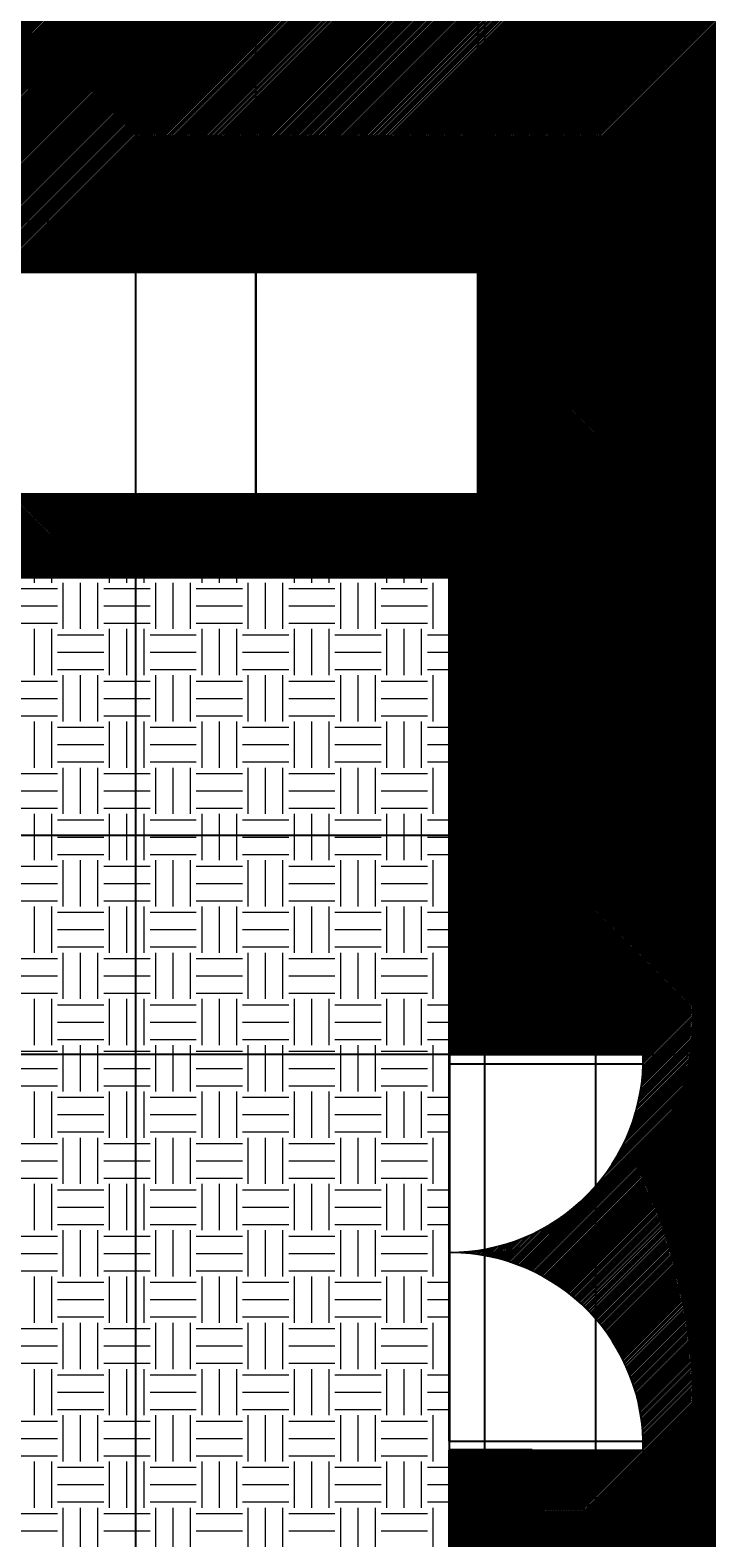
# Model space of a CAD drawing. Units: inches. Extents: x 205 to 1667, y -23 to 828.
# Tile 3 of 10: x 572 to 645, y 101 to 264. Entities that reach past the tile are written whole.
import ezdxf

# ---------------------------------------------------------------- set-up
doc = ezdxf.new("R2010")
doc.units = ezdxf.units.IN
doc.header["$MEASUREMENT"] = 0
for name, color, linetype, lineweight in [('A-ANNO-DIMS', 2, 'Continuous', 18), ('A-DOOR', 4, 'Continuous', 25), ('A-FLOR-CASE', 32, 'Continuous', 25), ('A-WALL', 7, 'Continuous', 35)]:
    doc.layers.add(name, color=color, linetype=linetype, lineweight=lineweight)
doc.layers.add('A-FLOR-PATT', color=9, linetype='Continuous', lineweight=9, true_color=0xc7c8ca)
doc.styles.get("Standard").update_dxf_attribs({"font": 'arial.ttf'})
doc.dimstyles.get("Standard").update_dxf_attribs({"dimtxt": 0.18, "dimasz": 0.18, "dimexe": 0.18, "dimexo": 0.0625, "dimgap": 0.09, "dimtad": 0, "dimtih": 1, "dimtoh": 1, "dimdec": 4, "dimzin": 0, "dimdsep": 46, "dimtxsty": 'Standard', "dimcen": 0.09, "dimadec": 0, "dimazin": 0, "dimtfac": 1, "dimtdec": 4, "dimtofl": 0, "dimtmove": 0, "dimatfit": 3, "dimfxl": 1, "dimtolj": 1, "dimtzin": 0, "dimarcsym": 0})

# ---------------------------------------------------------------- blocks, each defined once
blk = doc.blocks.new('DOOR-PAIR-21IN-LEAVES')
for p, q in [((0, 42.78), (0, 41.78)), ((0, 42.78), (21, 42.78)), ((0, 41.78), (21, 41.78)), ((0, 1), (0, 0)), ((0, 1), (21, 1)), ((0, 0), (21, 0))]:
    blk.add_line(p, q)
for centre, start, end in [((0.11, 42.28), 269.6873, 1.3714), ((0.11, 0.5), 358.6286, 89.6873)]:
    blk.add_arc(centre, 20.89, start, end)
blk = doc.blocks.new('*D19')
at = {"layer": 'A-ANNO-DIMS', "color": 0, "lineweight": -2, "transparency": 16777216}
for p, q in [((570, 213.93), (577.32, 213.93)), ((577.14, 213.75), (577.14, 209.61)), ((577.14, 205.11), (577.14, 209.25)), ((570, 204.93), (577.32, 204.93))]:
    blk.add_line(p, q, dxfattribs=at)
at = {"layer": 'A-ANNO-DIMS', "color": 0, "transparency": 16777216}
for points in [[(577.11, 213.75), (577.17, 213.75), (577.14, 213.93)], [(577.11, 205.11), (577.17, 205.11), (577.14, 204.93)]]:
    blk.add_solid(points, dxfattribs=at)
at = {"layer": 'Defpoints', "color": 0, "transparency": 16777216}
for p in [(569.94, 213.93), (577.14, 213.93), (569.94, 204.93)]:
    blk.add_point(p, dxfattribs=at)
at = {"layer": 'A-ANNO-DIMS', "color": 0, "transparency": 16777216, "insert": (577.14, 209.43), "char_height": 0.18, "attachment_point": 5}
blk.add_mtext('\\A1;9 TYP.', dxfattribs=at)
blk = doc.blocks.new('*D34')
at = {"layer": 'A-ANNO-DIMS', "color": 0, "lineweight": -2, "transparency": 16777216}
for p, q in [((638.54, 153.38), (645.08, 153.38)), ((644.9, 153.2), (644.9, 132.17)), ((644.9, 110.77), (644.9, 131.8)), ((638.54, 110.59), (645.08, 110.59))]:
    blk.add_line(p, q, dxfattribs=at)
at = {"layer": 'A-ANNO-DIMS', "color": 0, "transparency": 16777216}
for points in [[(644.87, 153.2), (644.93, 153.2), (644.9, 153.38)], [(644.87, 110.77), (644.93, 110.77), (644.9, 110.59)]]:
    blk.add_solid(points, dxfattribs=at)
at = {"layer": 'Defpoints', "color": 0, "transparency": 16777216}
for p in [(638.48, 153.38), (644.9, 153.38), (638.48, 110.59)]:
    blk.add_point(p, dxfattribs=at)
at = {"layer": 'A-ANNO-DIMS', "color": 0, "transparency": 16777216, "insert": (644.9, 131.98), "char_height": 0.18, "attachment_point": 5}
blk.add_mtext('\\A1;PAIRED DOOR 43', dxfattribs=at)
blk = doc.blocks.new('*D35')
at = {"layer": 'A-ANNO-DIMS', "color": 0, "lineweight": -2, "transparency": 16777216}
for p, q in [((617.35, 110.53), (617.35, 103.99)), ((638.48, 110.53), (638.48, 103.99)), ((617.53, 104.17), (627.71, 104.17)), ((638.3, 104.17), (628.12, 104.17))]:
    blk.add_line(p, q, dxfattribs=at)
at = {"layer": 'A-ANNO-DIMS', "color": 0, "transparency": 16777216}
for points in [[(617.53, 104.2), (617.53, 104.14), (617.35, 104.17)], [(638.3, 104.2), (638.3, 104.14), (638.48, 104.17)]]:
    blk.add_solid(points, dxfattribs=at)
at = {"layer": 'Defpoints', "color": 0, "transparency": 16777216}
for p in [(617.35, 110.59), (638.48, 110.59), (638.48, 104.17)]:
    blk.add_point(p, dxfattribs=at)
at = {"layer": 'A-ANNO-DIMS', "color": 0, "transparency": 16777216, "insert": (627.91, 104.17), "char_height": 0.18, "attachment_point": 5}
blk.add_mtext('\\A1;21', dxfattribs=at)
blk = doc.blocks.new('*D55')
at = {"layer": 'A-ANNO-DIMS', "color": 0, "lineweight": -2, "transparency": 16777216}
for p, q in [((621.22, 16.71), (621.22, 637.89)), ((621.4, 637.71), (627.01, 637.71)), ((633.04, 637.71), (627.43, 637.71)), ((633.22, 16.71), (633.22, 637.89))]:
    blk.add_line(p, q, dxfattribs=at)
at = {"layer": 'A-ANNO-DIMS', "color": 0, "transparency": 16777216}
for points in [[(621.4, 637.74), (621.4, 637.68), (621.22, 637.71)], [(633.04, 637.74), (633.04, 637.68), (633.22, 637.71)]]:
    blk.add_solid(points, dxfattribs=at)
at = {"layer": 'Defpoints', "color": 0, "transparency": 16777216}
for p in [(633.22, 637.71), (621.22, 16.65), (633.22, 16.65)]:
    blk.add_point(p, dxfattribs=at)
at = {"layer": 'A-ANNO-DIMS', "color": 0, "transparency": 16777216, "insert": (627.22, 637.71), "char_height": 0.18, "attachment_point": 5}
blk.add_mtext('\\A1;12', dxfattribs=at)
blk = doc.blocks.new('*D64')
at = {"layer": 'A-ANNO-DIMS', "color": 0, "lineweight": -2, "transparency": 16777216}
for p, q in [((471.43, 454.59), (471.43, -22.59)), ((583.44, 454.59), (583.44, -22.59)), ((471.61, -22.41), (527.16, -22.41)), ((583.26, -22.41), (527.71, -22.41))]:
    blk.add_line(p, q, dxfattribs=at)
at = {"layer": 'A-ANNO-DIMS', "color": 0, "transparency": 16777216}
for points in [[(471.61, -22.38), (471.61, -22.44), (471.43, -22.41)], [(583.26, -22.38), (583.26, -22.44), (583.44, -22.41)]]:
    blk.add_solid(points, dxfattribs=at)
at = {"layer": 'Defpoints', "color": 0, "transparency": 16777216}
for p in [(471.43, 454.65), (583.44, 454.65), (583.44, -22.41)]:
    blk.add_point(p, dxfattribs=at)
at = {"layer": 'A-ANNO-DIMS', "color": 0, "transparency": 16777216, "insert": (527.44, -22.41), "char_height": 0.18, "attachment_point": 5}
blk.add_mtext('\\A1;112', dxfattribs=at)
blk = doc.blocks.new('*D65')
at = {"layer": 'A-ANNO-DIMS', "color": 0, "lineweight": -2, "transparency": 16777216}
for p, q in [((617.28, 204.93), (432.19, 204.93)), ((432.37, 204.75), (432.37, 179.34)), ((432.37, 153.56), (432.37, 178.97)), ((617.28, 153.38), (432.19, 153.38))]:
    blk.add_line(p, q, dxfattribs=at)
at = {"layer": 'A-ANNO-DIMS', "color": 0, "transparency": 16777216}
for points in [[(432.34, 204.75), (432.4, 204.75), (432.37, 204.93)], [(432.34, 153.56), (432.4, 153.56), (432.37, 153.38)]]:
    blk.add_solid(points, dxfattribs=at)
at = {"layer": 'Defpoints', "color": 0, "transparency": 16777216}
for p in [(432.37, 204.93), (617.35, 204.93), (617.35, 153.38)]:
    blk.add_point(p, dxfattribs=at)
at = {"layer": 'A-ANNO-DIMS', "color": 0, "transparency": 16777216, "insert": (432.37, 179.15), "char_height": 0.18, "attachment_point": 5}
blk.add_mtext('\\A1;51.56', dxfattribs=at)
blk = doc.blocks.new('*D67')
at = {"layer": 'A-ANNO-DIMS', "color": 0, "lineweight": -2, "transparency": 16777216}
for p, q in [((691.44, 243.44), (432.19, 243.44)), ((432.37, 243.26), (432.37, 210.43)), ((432.37, 177.23), (432.37, 210.06)), ((691.44, 177.05), (432.19, 177.05))]:
    blk.add_line(p, q, dxfattribs=at)
at = {"layer": 'A-ANNO-DIMS', "color": 0, "transparency": 16777216}
for points in [[(432.34, 243.26), (432.4, 243.26), (432.37, 243.44)], [(432.34, 177.23), (432.4, 177.23), (432.37, 177.05)]]:
    blk.add_solid(points, dxfattribs=at)
at = {"layer": 'Defpoints', "color": 0, "transparency": 16777216}
for p in [(432.37, 243.44), (691.51, 243.44), (691.51, 177.05)]:
    blk.add_point(p, dxfattribs=at)
at = {"layer": 'A-ANNO-DIMS', "color": 0, "transparency": 16777216, "insert": (432.37, 210.24), "char_height": 0.18, "attachment_point": 5}
blk.add_mtext('\\A1;66.39', dxfattribs=at)
blk = doc.blocks.new('*D68')
at = {"layer": 'A-ANNO-DIMS', "color": 0, "lineweight": -2, "transparency": 16777216}
for p, q in [((626.35, 153.44), (626.35, 637.89)), ((626.53, 637.71), (658.53, 637.71)), ((691.33, 637.71), (659.32, 637.71)), ((691.51, 177.11), (691.51, 637.89))]:
    blk.add_line(p, q, dxfattribs=at)
at = {"layer": 'A-ANNO-DIMS', "color": 0, "transparency": 16777216}
for points in [[(626.53, 637.74), (626.53, 637.68), (626.35, 637.71)], [(691.33, 637.74), (691.33, 637.68), (691.51, 637.71)]]:
    blk.add_solid(points, dxfattribs=at)
at = {"layer": 'Defpoints', "color": 0, "transparency": 16777216}
for p in [(626.35, 637.71), (691.51, 177.05), (626.35, 153.38)]:
    blk.add_point(p, dxfattribs=at)
at = {"layer": 'A-ANNO-DIMS', "color": 0, "transparency": 16777216, "insert": (658.93, 637.71), "char_height": 0.18, "attachment_point": 5}
blk.add_mtext('\\A1;65.16', dxfattribs=at)
blk = doc.blocks.new('*D80')
at = {"layer": 'A-ANNO-DIMS', "color": 0, "lineweight": -2, "transparency": 16777216}
for p, q in [((596.44, 213.99), (596.44, 637.89)), ((596.62, 637.71), (608.22, 637.71)), ((620.26, 637.71), (608.66, 637.71)), ((620.44, 213.99), (620.44, 637.89))]:
    blk.add_line(p, q, dxfattribs=at)
at = {"layer": 'A-ANNO-DIMS', "color": 0, "transparency": 16777216}
for points in [[(596.62, 637.74), (596.62, 637.68), (596.44, 637.71)], [(620.26, 637.74), (620.26, 637.68), (620.44, 637.71)]]:
    blk.add_solid(points, dxfattribs=at)
at = {"layer": 'Defpoints', "color": 0, "transparency": 16777216}
for p in [(596.44, 637.71), (596.44, 213.93), (620.44, 213.93)]:
    blk.add_point(p, dxfattribs=at)
at = {"layer": 'A-ANNO-DIMS', "color": 0, "transparency": 16777216, "insert": (608.44, 637.71), "char_height": 0.18, "attachment_point": 5}
blk.add_mtext('\\A1;24', dxfattribs=at)
blk = doc.blocks.new('*D81')
at = {"layer": 'A-ANNO-DIMS', "color": 0, "lineweight": -2, "transparency": 16777216}
for p, q in [((596.38, 237.93), (432.19, 237.93)), ((432.37, 237.75), (432.37, 226.11)), ((432.37, 214.11), (432.37, 225.75)), ((596.38, 213.93), (432.19, 213.93))]:
    blk.add_line(p, q, dxfattribs=at)
at = {"layer": 'A-ANNO-DIMS', "color": 0, "transparency": 16777216}
for points in [[(432.34, 237.75), (432.4, 237.75), (432.37, 237.93)], [(432.34, 214.11), (432.4, 214.11), (432.37, 213.93)]]:
    blk.add_solid(points, dxfattribs=at)
at = {"layer": 'Defpoints', "color": 0, "transparency": 16777216}
for p in [(432.37, 237.93), (596.44, 237.93), (596.44, 213.93)]:
    blk.add_point(p, dxfattribs=at)
at = {"layer": 'A-ANNO-DIMS', "color": 0, "transparency": 16777216, "insert": (432.37, 225.93), "char_height": 0.18, "attachment_point": 5}
blk.add_mtext('\\A1;24', dxfattribs=at)

msp = doc.modelspace()

# ---------------------------------------------------------------- hatches: boundary and pattern name
at = {"layer": 'A-FLOR-PATT'}
h = msp.add_hatch(dxfattribs=at)
h.set_pattern_fill('ANSI31', color=256)
h.paths.add_polyline_path([(774.4305, 607.6511), (720.5338, 607.6511), (720.5338, 598.6511), (727.9933, 598.6511), (746.8614, 598.6511), (765.4305, 598.6511), (765.4305, 454.6511), (759.5298, 454.6511), (759.5298, 448.9635), (765.4305, 448.9635), (765.4305, 428.0602), (774.4305, 428.0602)])
h.paths.add_polyline_path([(765.4305, 598.6511), (746.8614, 598.6511), (746.8614, 579.7829), (727.9933, 579.7829), (727.9933, 518.1387, -0.41421701), (724.6389, 514.7843), (668.2693, 514.7843, -0.41421356), (665.0743, 517.9793), (665.0743, 579.7829), (646.2062, 579.7829), (646.2062, 598.6511), (626.3468, 598.6511), (626.3468, 454.6511), (628.3468, 454.6511), (628.3468, 484.9635, -0.41421356), (664.3468, 449.9635), (664.3468, 454.6511), (729.3305, 454.6511), (758.5298, 454.6511), (759.5298, 454.6511), (765.4305, 454.6511)])
h.paths.add_polyline_path([(621.4404, 598.6511), (471.4305, 598.6511), (471.4305, 568.8442), (490.2987, 568.8442), (490.2987, 549.9761), (551.9429, 549.9761, -0.41421701), (555.2973, 546.6217), (555.2973, 490.2521, -0.41421356), (552.1023, 487.0571), (490.2987, 487.0571), (490.2987, 468.189), (471.4305, 468.189), (471.4305, 454.6511), (583.4404, 454.6511), (583.4404, 449.9635, -0.41421356), (619.4404, 484.9635), (619.4404, 454.6511), (621.4404, 454.6511)])
h.paths.add_polyline_path([(672.5338, 607.6511), (569.5707, 607.6511), (569.5707, 598.6511), (621.4404, 598.6511), (621.4404, 454.6511), (619.4404, 454.6511), (619.4404, 448.9635), (628.3468, 448.9635), (628.3468, 454.6511), (626.3468, 454.6511), (626.3468, 598.6511), (646.2062, 598.6511), (665.0743, 598.6511), (672.5338, 598.6511)])
h.paths.add_polyline_path([(521.5707, 607.6511), (462.4305, 607.6511), (462.4305, 407.4306), (471.4305, 407.4306), (471.4305, 448.9635), (583.4404, 448.9635, -0.0070419), (583.4404, 449.9635), (583.4404, 454.6511), (471.4305, 454.6511), (471.4305, 468.189), (471.4305, 487.0571), (471.4305, 549.9761), (471.4305, 568.8442), (471.4305, 598.6511), (521.5707, 598.6511)])
h.paths.add_polyline_path([(471.4305, 314.3187), (583.4404, 314.3187), (583.4404, 319.9388), (471.4305, 319.9388), (471.4305, 359.4306), (462.4305, 359.4306), (462.4305, 7.6511), (471.4305, 7.6511), (471.4305, 204.9321), (521.9355, 204.9321), (521.9355, 213.9321), (471.4305, 213.9321)])
h.paths.add_polyline_path([(774.4305, 410.0602), (765.4305, 410.0602), (765.4305, 389.1569), (672.3024, 389.1569), (672.3024, 448.9635), (681.1739, 448.9635, -0.18532444), (681.6564, 449.1487), (698.6035, 449.1487), (729.3305, 448.9635), (729.3305, 454.6511), (664.3468, 454.6511), (664.3468, 449.9635, -0.0070419), (664.3468, 448.9635), (666.3024, 448.9635), (666.3024, 378.2485), (672.3024, 378.2485), (672.3024, 383.1306), (765.4305, 383.1306), (765.4305, 360.5347), (774.4305, 360.5347)])
h.paths.add_polyline_path([(774.4305, 342.5347), (765.4305, 342.5347), (765.4305, 319.9388), (672.3024, 319.9388), (672.3024, 348.5574), (671.0896, 348.5574, -0.04071533), (666.3024, 348.2485), (666.3024, 319.9388), (664.3468, 319.9388, -0.0070419), (664.3468, 318.9388), (664.3468, 314.3187), (765.4305, 314.3187), (765.4305, 290.8426), (774.4305, 290.8426)])
h.paths.add_polyline_path([(774.4305, 242.8426), (765.4305, 242.8426), (765.4305, 104.6382), (626.3468, 104.6382), (626.3468, 110.5917), (617.3468, 110.5917), (617.3468, 95.6382), (765.4305, 95.6382), (765.4305, 16.6511), (621.2232, 16.6511), (621.2232, 7.6511), (774.4305, 7.6511)])
h.paths.add_polyline_path([(626.3468, 314.3187), (628.3468, 314.3187), (628.3468, 319.9388), (619.4404, 319.9388), (619.4404, 314.3187), (620.4404, 314.3187), (620.4404, 213.9321), (569.9355, 213.9321), (569.9355, 204.9321), (617.3468, 204.9321), (617.3468, 153.3751), (626.3468, 153.3751)])
h.paths.add_polyline_path([(620.4404, 314.3187), (619.4404, 314.3187), (619.4404, 319.9388), (628.3468, 319.9388), (629.3468, 319.9388), (629.3468, 283.9388, 0.40598745), (664.3468, 318.9388), (664.3468, 319.9388), (666.3024, 319.9388), (666.3024, 348.2485), (666.3024, 377.2485), (666.3024, 378.2485), (666.3024, 448.9635), (664.3468, 448.9635), (664.3468, 449.9635, 0.40598745), (629.3468, 484.9635), (629.3468, 448.9635), (628.3468, 448.9635), (619.4404, 448.9635), (618.4404, 448.9635), (618.4404, 484.9635, 0.40598745), (583.4404, 449.9635), (583.4404, 448.9635), (471.4305, 448.9635), (471.4305, 407.4306), (471.4305, 359.4306), (471.4305, 319.9388), (583.4404, 319.9388), (583.4404, 314.3187), (495.4305, 314.3187), (495.4305, 237.9321), (620.4404, 237.9321)])
h.paths.add_polyline_path([(525.0876, 347.7863), (513.5657, 347.7863), (512.0216, 362.1672), (526.6317, 362.1672)], flags=16)
h.paths.add_polyline_path([(550.9499, 370.1471), (536.569, 368.6029), (536.569, 383.2131), (550.9499, 381.6689)], flags=16)
h.paths.add_polyline_path([(530.7713, 364.5431), (508.0415, 364.5431, -0.41421356), (504.7944, 367.7902), (504.7944, 403.5085, -0.41421356), (508.0415, 406.7556), (530.7713, 406.7556, -0.41421356), (534.0184, 403.5085), (534.0184, 367.7902, -0.41421356)], flags=16)
h.paths.add_polyline_path([(550.9499, 389.6298), (536.569, 388.0856), (536.569, 402.6958), (550.9499, 401.1516)], flags=16)
h.paths.add_polyline_path([(502.2439, 368.6029), (487.863, 370.1471), (487.863, 381.6689), (502.2439, 383.2131)], flags=16)
h.paths.add_polyline_path([(502.2439, 388.0856), (487.863, 389.6298), (487.863, 401.1516), (502.2439, 402.6958)], flags=16)
h.paths.add_polyline_path([(526.6317, 409.1315), (512.0216, 409.1315), (513.5657, 423.5124), (525.0876, 423.5124)], flags=16)
h.paths.add_polyline_path([(765.4305, 290.8426), (765.4305, 314.3187), (664.3468, 314.3187), (664.3468, 318.9388, -0.41421356), (628.3468, 283.9388), (628.3468, 314.3187), (626.3468, 314.3187), (626.3468, 153.3751), (638.3468, 153.3751, -0.4196361), (617.5748, 131.9834, -0.4196361), (638.3468, 110.5917), (626.3468, 110.5917), (626.3468, 104.6382), (765.4305, 104.6382), (765.4305, 242.8426)])
h.paths.add_polyline_path([(691.5064, 243.4363), (693.2483, 243.4363), (725.4984, 243.4363), (725.4984, 241.7329), (725.4984, 177.0512), (723.7564, 177.0512), (691.5064, 177.0512), (691.5064, 178.7545)], flags=16)
h.paths.add_polyline_path([(689.8658, 265.2977), (689.8658, 296.6873, -0.41421356), (690.8346, 297.6561), (724.6111, 297.6561, -0.41421356), (725.5799, 296.6873), (725.5799, 265.2977, -0.41421356), (724.6111, 264.3289), (690.8346, 264.3289, -0.41421356)], flags=16)
h.paths.add_polyline_path([(694.1286, 265.6852), (694.1286, 288.9368, -0.41421356), (695.0974, 289.9056), (720.3483, 289.9056, -0.41421356), (721.3171, 288.9368), (721.3171, 265.6852, -0.04533947), (721.3013, 265.5106, -0.3531705), (720.3282, 264.7164), (695.0974, 264.7164, -0.41421356)], flags=0)
h.paths.add_polyline_path([(694.1286, 291.2619), (694.1286, 294.7497, -0.41421356), (695.0974, 295.7185), (720.3483, 295.7185, -0.41421356), (721.3171, 294.7497), (721.3171, 291.2619, -0.41421356), (720.3483, 290.2931), (695.0974, 290.2931, -0.41421356)], flags=0)
h.paths.add_polyline_path([(734.4369, 244.6615, -0.41421356), (735.2682, 245.4928), (762.2019, 245.4928, -0.41421356), (763.0332, 244.6615), (763.0332, 168.183, -0.41421356), (762.2019, 167.3517), (735.2682, 167.3517, -0.41421356), (734.4369, 168.183)], flags=16)
h.paths.add_polyline_path([(761.7032, 242.1676), (761.7032, 170.6768), (735.6007, 171.0093, -0.41421356), (734.7694, 171.8406), (734.7694, 193.5102, -0.56972741), (735.6007, 194.674, -0.41421356), (734.7694, 195.5053), (734.7694, 217.3423, -0.56972741), (735.6007, 218.5061, -0.41421356), (734.7694, 219.3374), (734.7694, 241.0038, -0.41421356), (735.6007, 241.8351), (735.1643, 242.1676)], flags=16)
h.paths.add_polyline_path([(757.5467, 171.0093), (760.5393, 171.0093, 0.41421356), (761.3706, 171.8406), (761.3706, 193.5102, 0.41421356), (760.5393, 194.3415), (757.5467, 194.3415, 0.41421356), (756.7154, 193.5102), (756.7155, 171.8534, 0.41871477)], flags=0)
h.paths.add_polyline_path([(756.7154, 241.0038, -0.41421356), (757.5467, 241.8351), (760.5393, 241.8351, -0.41421356), (761.3706, 241.0038), (761.3706, 219.3374, -0.41421356), (760.5393, 218.5061), (760.5393, 218.1736, -0.41421356), (761.3706, 217.3423), (761.3706, 195.5053, -0.41421356), (760.5393, 194.674), (757.5467, 194.674, -0.56972741), (756.3829, 195.5053, -0.41421356), (755.5516, 194.674), (755.5516, 194.3415, -0.41421356), (756.3829, 193.5102), (756.7154, 171.8406), (756.3829, 193.5102, 0.41421356), (755.5516, 194.3415), (735.6007, 194.674), (755.5516, 194.674, 0.41421356), (756.3829, 195.5053), (756.3829, 217.3423, 0.41421356), (755.5516, 218.1736), (735.6007, 218.5061), (755.5516, 218.5061, 0.41421356), (756.3829, 219.3374)], flags=0)
h.paths.add_polyline_path([(694.5151, 150.3608), (728.2916, 150.3608, -0.41421356), (729.2604, 149.3919), (729.2604, 118.0023, -0.41421356), (728.2916, 117.0335), (694.5151, 117.0335, -0.41421356), (693.5463, 118.0023), (693.5463, 149.3919, -0.41421356)], flags=16)
h.paths.add_polyline_path([(724.0288, 149.9732, -0.41421356), (724.9977, 149.0044), (724.9977, 125.7529, -0.41421356), (724.0288, 124.784), (698.7779, 124.784, -0.41421356), (697.8091, 125.7529), (697.8091, 149.0044, -0.04533947), (697.825, 149.179, -0.3531705), (698.798, 149.9732)], flags=0)
h.paths.add_polyline_path([(698.7779, 124.3965), (724.0288, 124.3965, -0.41421356), (724.9977, 123.4277), (724.9977, 119.94, -0.41421356), (724.0288, 118.9711), (698.7779, 118.9711, -0.41421356), (697.8091, 119.94), (697.8091, 123.4277, -0.41421356)], flags=0)
h = msp.add_hatch(dxfattribs=at)
h.set_pattern_fill('EARTH', color=256, scale=20)
h.paths.add_polyline_path([(617.3468, 204.9321), (471.4305, 204.9321), (471.4305, 7.6511), (621.2232, 7.6511), (621.2232, 95.6382), (617.3468, 95.6382), (617.3468, 110.5917), (617.3468, 111.5917)])
h.paths.add_polyline_path([(564.1913, 176.2169), (561.5098, 174.5217), (562.5, 170.769), (563.5731, 169.029), (563.5731, 147.7805), (563.1483, 146.2164), (563.1483, 96.7087), (563.8223, 94.5214), (563.8223, 70.9058), (562.7294, 70.1011), (562.6164, 59.3401), (563.5441, 58.4056), (563.5465, 55.9057), (561.4952, 53.5377), (552.1213, 53.5377), (551.0475, 54.9563), (550.7331, 57.4626), (541.3672, 57.4626), (532.0012, 57.4626), (531.6868, 54.9563), (530.613, 53.5377), (521.2392, 53.5377), (519.1879, 55.9057), (519.1903, 58.4056), (520.1179, 59.3401), (520.0049, 70.1011), (518.912, 70.9058), (518.912, 94.5214), (519.5861, 96.7087), (519.5861, 146.2164), (519.1613, 147.7805), (519.1613, 169.029), (520.2343, 170.769), (521.2245, 174.5217), (518.5431, 176.2169), (518.8594, 180.2791), (522.745, 182.0164), (541.3672, 182.0164), (559.9894, 182.0164), (563.8749, 180.2791)], flags=16)
h.paths.add_polyline_path([(553.7175, 178.3241), (557.6423, 162.0145), (557.6609, 142.4613), (541.3672, 143.5621), (525.0735, 142.4613), (525.092, 162.0145), (529.0169, 178.3241), (530.7323, 178.2589), (541.3672, 179.0078), (552.002, 178.2589)], flags=0)
h.paths.add_polyline_path([(560.4781, 137.464), (559.7214, 135.1419), (555.0412, 127.459), (552.6762, 126.3854), (546.7369, 128.3886), (541.3672, 128.3886), (535.9975, 128.3886), (530.0582, 126.3854), (527.6931, 127.459), (523.013, 135.1419), (522.2563, 137.464), (527.3921, 139.5127), (541.3672, 141.5088), (555.3423, 139.5127)], flags=0)
h.paths.add_polyline_path([(559.8869, 130.9684), (559.8869, 109.832), (556.6594, 109.832), (556.6594, 68.7114), (555.1011, 64.335), (552.6025, 63.0718), (541.3672, 63.0718), (530.1319, 63.0718), (527.6333, 64.335), (526.075, 68.7114), (526.075, 109.832), (522.8474, 109.832), (522.8474, 130.9684), (525.3715, 127.1487), (526.075, 122.4588), (526.075, 68.7114), (527.6333, 64.335), (530.1319, 63.0718), (541.3672, 63.0718), (552.6025, 63.0718), (555.1011, 64.335), (556.6594, 68.7114), (556.6594, 122.4588), (557.3629, 127.1487)], flags=0)
h.paths.add_polyline_path([(553.3621, 61.1985), (554.9264, 60.2724), (553.8564, 58.7089), (542.7405, 58.6984), (542.1147, 59.6353), (542.9167, 61.1985)], flags=0)
h.paths.add_polyline_path([(539.8176, 61.1985), (540.6197, 59.6353), (539.9938, 58.6984), (528.8779, 58.7089), (527.808, 60.2724), (529.3722, 61.1985)], flags=0)

# ---------------------------------------------------------------- linework, layer by layer
at = {"layer": 'A-FLOR-CASE'}
for p, q in [((620.4404, 237.9321), (495.4305, 237.9321)), ((596.4404, 237.9321), (596.4404, 213.9321))]:
    msp.add_line(p, q, dxfattribs=at)
at = {"layer": 'A-WALL'}
for p, q in [((620.4404, 314.3187), (620.4404, 213.9321)), ((626.3468, 314.3187), (626.3468, 153.3751)), ((620.4404, 213.9321), (471.4305, 213.9321)), ((617.3468, 204.9321), (471.4305, 204.9321)), ((617.3468, 204.9321), (617.3468, 111.5917)), ((626.3468, 153.3751), (617.3468, 153.3751)), ((626.3468, 110.5917), (617.3468, 110.5917)), ((617.3468, 110.5917), (617.3468, 95.6382)), ((626.3468, 110.5917), (626.3468, 104.6382)), ((765.4305, 104.6382), (626.3468, 104.6382))]:
    msp.add_line(p, q, dxfattribs=at)

# ---------------------------------------------------------------- block references
at = {"layer": 'A-DOOR'}
msp.add_blockref('DOOR-PAIR-21IN-LEAVES', (617.347, 110.592), dxfattribs=at)

# ---------------------------------------------------------------- dimensions: what is measured, and where the dimension line sits
at = {"layer": 'A-ANNO-DIMS'}
for base, p1, p2, override, picture, middle in [((596.4404, 637.7086), (620.4404, 213.9321), (596.4404, 213.9321), {"dimdec": 0, "dimlfac": 1, "dimrnd": 0, "dimzin": 0, "dimdsep": 46, "dimlunit": 2}, '*D80', (608.4404, 637.7086)), ((633.2232, 637.7086), (621.2232, 16.6511), (633.2232, 16.6511), {"dimdec": 0, "dimlfac": 1, "dimrnd": 0, "dimzin": 0, "dimdsep": 46, "dimlunit": 2}, '*D55', (627.2232, 637.7086)), ((626.3468, 637.7086), (691.5064, 177.0512), (626.3468, 153.3751), {"dimdec": 2, "dimlfac": 1, "dimrnd": 0, "dimzin": 0, "dimdsep": 46, "dimlunit": 2}, '*D68', (658.9266, 637.7086)), ((583.4404, -22.4064), (471.4305, 454.6511), (583.4404, 454.6511), {"dimdec": 0, "dimlfac": 1, "dimrnd": 0, "dimzin": 0, "dimdsep": 46, "dimlunit": 2}, '*D64', (527.4355, -22.4064)), ((638.4819, 104.1742), (617.3468, 110.5917), (638.4819, 110.5917), {"dimdec": 0, "dimlfac": 1, "dimrnd": 0, "dimzin": 0, "dimdsep": 46, "dimlunit": 2}, '*D35', (627.9143, 104.1742))]:
    dim = msp.add_linear_dim(base=base, p1=p1, p2=p2, dimstyle='Standard', override=override, dxfattribs=at)
    dim.commit()
    dim.dimension.update_dxf_attribs({"geometry": picture, "text_midpoint": middle})
for base, p1, p2, override, picture, middle in [((432.3731, 243.4363), (691.5064, 177.0512), (691.5064, 243.4363), {"dimdec": 2, "dimlfac": 1, "dimrnd": 0, "dimzin": 0, "dimdsep": 46, "dimlunit": 2}, '*D67', (432.3731, 210.2437)), ((432.3731, 237.9321), (596.4404, 213.9321), (596.4404, 237.9321), {"dimdec": 0, "dimlfac": 1, "dimrnd": 0, "dimzin": 0, "dimdsep": 46, "dimlunit": 2}, '*D81', (432.3731, 225.9321)), ((432.3731, 204.9321), (617.3468, 153.3751), (617.3468, 204.9321), {"dimdec": 2, "dimlfac": 1, "dimrnd": 0, "dimzin": 0, "dimdsep": 46, "dimlunit": 2}, '*D65', (432.3731, 179.1536))]:
    dim = msp.add_linear_dim(base=base, p1=p1, p2=p2, angle=90, dimstyle='Standard', override=override, dxfattribs=at)
    dim.commit()
    dim.dimension.update_dxf_attribs({"geometry": picture, "text_midpoint": middle})
for base, p1, p2, text, picture, middle in [((577.1355, 213.9321), (569.9355, 204.9321), (569.9355, 213.9321), '<> TYP.', '*D19', (577.1355, 209.4321)), ((644.8994, 153.3751), (638.4819, 110.5917), (638.4819, 153.3751), 'PAIRED DOOR <>', '*D34', (644.8994, 131.9834))]:
    dim = msp.add_linear_dim(base=base, p1=p1, p2=p2, angle=90, text=text, dimstyle='Standard', override={"dimdec": 0, "dimlfac": 1, "dimrnd": 0, "dimzin": 0, "dimdsep": 46, "dimlunit": 2}, dxfattribs=at)
    dim.commit()
    dim.dimension.update_dxf_attribs({"geometry": picture, "text_midpoint": middle})

doc.saveas('drawing.dxf')
